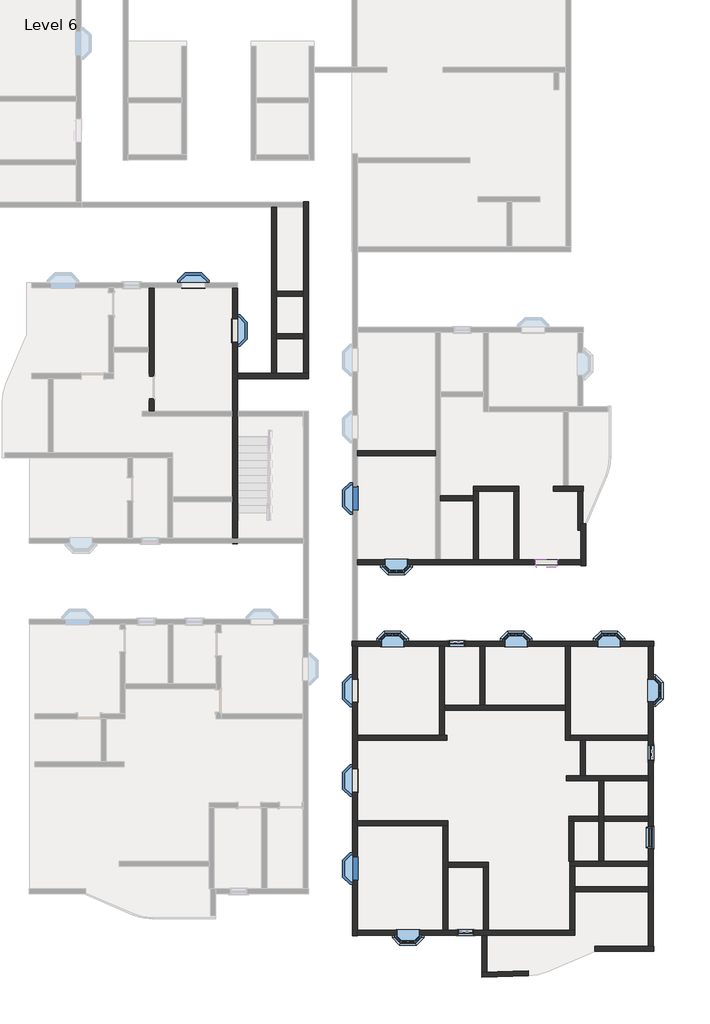
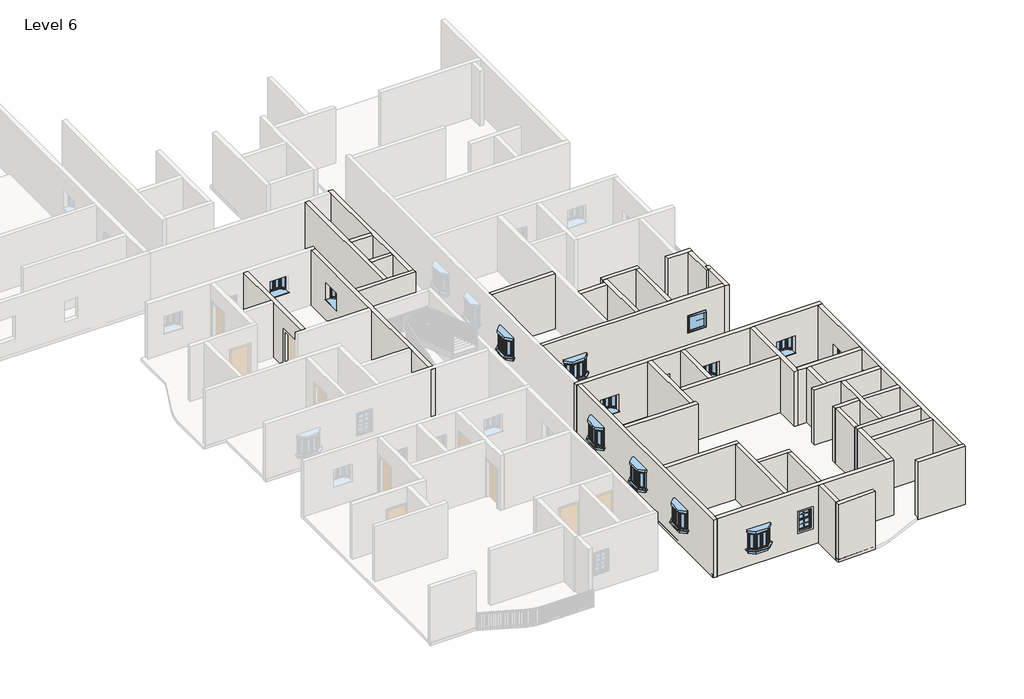
# One storey, part 2 of 14: 41 walls, 17 windows.
"""IFC4 building model written with IfcOpenShell, lengths in millimetres."""

from ifc_helpers import new_model, si_unit, frame, origin, place, context, project, spatial, polyline, outline, extrude, faceted_brep, transform, mapped, element, save
from components import window_910x910mm_67ef725a, window_8debb0fa, windows_sgl_w_glazing_bars_910x910mm_256712d0

model = new_model("IFC4")

# Units and contexts
model_context = context("Model", 3, world=origin())
ifc_project = project(units=[si_unit("LENGTHUNIT", "METRE", prefix="MILLI")], contexts=[model_context])

# Site, building, storey
site = spatial("IfcSite", under=ifc_project)
building = spatial("IfcBuilding", under=site)
storey = spatial("IfcBuildingStorey", under=building, Name="Level 6", Elevation=15240.0)

# Walls
placement = place(None, origin())
element("IfcWall", 1, ObjectType="4.5\" p", at=placement, inside=storey, context=model_context, shape_type="SweptSolid", body=[
    extrude(outline(polyline([(6070.4380523, -28284.6234353), (6070.4380523, -26796.6042694), (6273.6380523, -26796.6042694), (6273.6380523, -28277.5275349), (6070.4380523, -28284.6234353)])), frame((0.0, 0.0, 15240.0), z_axis=(0.0, 0.0, 1.0), x_axis=(1.0, 0.0, 0.0)), (0.0, 0.0, 1.0), 3048.0),
])
element("IfcWall", 2, ObjectType="4.5\" p", at=placement, inside=storey, context=model_context, shape_type="Brep", body=[
    faceted_brep([(6070.4380523, -28487.9472947, 15240.0), (7954.8443294, -28422.1423774, 15240.0), (7954.8443294, -28422.1423774, 18288.0), (6070.4380523, -28487.9472947, 18288.0), (6070.4380523, -28284.6234353, 15240.0), (6070.4380523, -28284.6234353, 18288.0), (6273.6380523, -28277.5275349, 18288.0), (7947.7527517, -28219.0661614, 18288.0), (7947.7527517, -28219.0661614, 15240.0), (6273.6380523, -28277.5275349, 15240.0)], [[[0, 1, 2, 3]], [[4, 5, 6, 7, 8, 9]], [[1, 0, 4, 9, 8]], [[2, 1, 8, 7]], [[3, 2, 7, 6, 5]], [[0, 3, 5, 4]]]),
])
element("IfcWall", 3, ObjectType="4.5\" p", at=placement, inside=storey, context=model_context, shape_type="Brep", body=[
    faceted_brep([(10639.6896214, -27431.6042694, 15240.0), (13030.0380523, -27431.6042694, 15240.0), (13030.0380523, -27431.6042694, 18288.0), (10639.6896214, -27431.6042694, 18288.0), (10639.6896214, -27228.4042694, 15240.0), (10639.6896214, -27228.4042694, 18288.0), (12814.1380523, -27228.4042694, 18288.0), (13017.3380523, -27228.4042694, 18288.0), (13030.0380523, -27228.4042694, 18288.0), (13030.0380523, -27228.4042694, 15240.0), (13017.3380523, -27228.4042694, 15240.0), (12814.1380523, -27228.4042694, 15240.0)], [[[0, 1, 2, 3]], [[4, 5, 6, 7, 8, 9, 10, 11]], [[1, 0, 4, 11, 10, 9]], [[2, 1, 9, 8]], [[3, 2, 8, 7, 6, 5]], [[0, 3, 5, 4]]]),
])
element("IfcWall", 4, ObjectType="4.5\" p", at=placement, inside=storey, context=model_context, shape_type="Brep", body=[
    faceted_brep([(1015.8380523, -18878.1542694, 15240.0), (4648.0380523, -18878.1542694, 15240.0), (4648.0380523, -18878.1542694, 18288.0), (1015.8380523, -18878.1542694, 18288.0), (1015.8380523, -18674.9542694, 15240.0), (1015.8380523, -18674.9542694, 18288.0), (4336.8880523, -18674.9542694, 18288.0), (4540.0880523, -18674.9542694, 18288.0), (4648.0380523, -18674.9542694, 18288.0), (4648.0380523, -18674.9542694, 15240.0), (4540.0880523, -18674.9542694, 15240.0), (4336.8880523, -18674.9542694, 15240.0)], [[[0, 1, 2, 3]], [[4, 5, 6, 7, 8, 9, 10, 11]], [[1, 0, 4, 11, 10, 9]], [[2, 1, 9, 8]], [[3, 2, 8, 7, 6, 5]], [[0, 3, 5, 4]]]),
])
element("IfcWall", 5, ObjectType="4.5\" p", at=placement, inside=storey, context=model_context, shape_type="Brep", body=[
    faceted_brep([(4336.8880523, -15049.1042694, 15240.0), (4336.8880523, -18674.9542694, 15240.0), (4336.8880523, -18674.9542694, 18288.0), (4336.8880523, -15049.1042694, 18288.0), (4540.0880523, -15049.1042694, 15240.0), (4540.0880523, -15049.1042694, 18288.0), (4540.0880523, -17455.7542694, 18288.0), (4540.0880523, -17658.9542694, 18288.0), (4540.0880523, -18674.9542694, 18288.0), (4540.0880523, -18674.9542694, 15240.0), (4540.0880523, -17658.9542694, 15240.0), (4540.0880523, -17455.7542694, 15240.0)], [[[0, 1, 2, 3]], [[4, 5, 6, 7, 8, 9, 10, 11]], [[1, 0, 4, 11, 10, 9]], [[3, 2, 8, 7, 6, 5]], [[0, 3, 5, 4]], [[2, 1, 9, 8]]]),
])
element("IfcWall", 6, ObjectType="4.5\" p", at=placement, inside=storey, context=model_context, shape_type="Brep", body=[
    faceted_brep([(4540.0880523, -17658.9542694, 15240.0), (9442.2880523, -17658.9542694, 15240.0), (9442.2880523, -17658.9542694, 18288.0), (4540.0880523, -17658.9542694, 18288.0), (4540.0880523, -17455.7542694, 15240.0), (4540.0880523, -17455.7542694, 18288.0), (5975.1880523, -17455.7542694, 18288.0), (6178.3880523, -17455.7542694, 18288.0), (9442.2880523, -17455.7542694, 18288.0), (9442.2880523, -17455.7542694, 15240.0), (6178.3880523, -17455.7542694, 15240.0), (5975.1880523, -17455.7542694, 15240.0)], [[[0, 1, 2, 3]], [[4, 5, 6, 7, 8, 9, 10, 11]], [[1, 0, 4, 11, 10, 9]], [[3, 2, 8, 7, 6, 5]], [[0, 3, 5, 4]], [[2, 1, 9, 8]]]),
])
element("IfcWall", 7, ObjectType="4.5\" p", at=placement, inside=storey, context=model_context, shape_type="SweptSolid", body=[
    extrude(outline(polyline([(5975.1880523, -17455.7542694), (5975.1880523, -15049.1042694), (6178.3880523, -15049.1042694), (6178.3880523, -17455.7542694), (5975.1880523, -17455.7542694)])), frame((0.0, 0.0, 15240.0), z_axis=(0.0, 0.0, 1.0), x_axis=(1.0, 0.0, 0.0)), (0.0, 0.0, 1.0), 3048.0),
])
element("IfcWall", 8, ObjectType="4.5\" p", at=placement, inside=storey, context=model_context, shape_type="Brep", body=[
    faceted_brep([(9442.2880523, -15049.1042694, 15240.0), (9442.2880523, -17455.7542694, 15240.0), (9442.2880523, -17658.9542694, 15240.0), (9442.2880523, -18871.8042694, 15240.0), (9442.2880523, -18871.8042694, 18288.0), (9442.2880523, -17658.9542694, 18288.0), (9442.2880523, -17455.7542694, 18288.0), (9442.2880523, -15049.1042694, 18288.0), (9645.4880523, -15049.1042694, 15240.0), (9645.4880523, -15049.1042694, 18288.0), (9645.4880523, -18668.6042694, 18288.0), (9645.4880523, -18871.8042694, 18288.0), (9645.4880523, -18871.8042694, 15240.0), (9645.4880523, -18668.6042694, 15240.0)], [[[0, 1, 2, 3, 4, 5, 6, 7]], [[8, 9, 10, 11, 12, 13]], [[3, 2, 1, 0, 8, 13, 12]], [[7, 6, 5, 4, 11, 10, 9]], [[0, 7, 9, 8]], [[4, 3, 12, 11]]]),
])
element("IfcWall", 9, ObjectType="4.5\" p", at=placement, inside=storey, context=model_context, shape_type="Brep", body=[
    faceted_brep([(1015.8380523, -22345.2542694, 15240.0), (4489.2880523, -22345.2542694, 15240.0), (4692.4880523, -22345.2542694, 15240.0), (4692.4880523, -22345.2542694, 18288.0), (4489.2880523, -22345.2542694, 18288.0), (1015.8380523, -22345.2542694, 18288.0), (1015.8380523, -22142.0542694, 15240.0), (1015.8380523, -22142.0542694, 18288.0), (4692.4880523, -22142.0542694, 18288.0), (4692.4880523, -22142.0542694, 15240.0)], [[[0, 1, 2, 3, 4, 5]], [[6, 7, 8, 9]], [[2, 1, 0, 6, 9]], [[5, 4, 3, 8, 7]], [[0, 5, 7, 6]], [[3, 2, 9, 8]]]),
])
element("IfcWall", 10, ObjectType="4.5\" p", at=placement, inside=storey, context=model_context, shape_type="Brep", body=[
    faceted_brep([(4489.2880523, -22345.2542694, 15240.0), (4489.2880523, -26580.7042694, 15240.0), (4489.2880523, -26580.7042694, 18288.0), (4489.2880523, -22345.2542694, 18288.0), (4692.4880523, -22345.2542694, 15240.0), (4692.4880523, -22345.2542694, 18288.0), (4692.4880523, -23818.4542694, 18288.0), (4692.4880523, -24021.6542694, 18288.0), (4692.4880523, -26580.7042694, 18288.0), (4692.4880523, -26580.7042694, 15240.0), (4692.4880523, -24021.6542694, 15240.0), (4692.4880523, -23818.4542694, 15240.0)], [[[0, 1, 2, 3]], [[4, 5, 6, 7, 8, 9, 10, 11]], [[1, 0, 4, 11, 10, 9]], [[3, 2, 8, 7, 6, 5]], [[0, 3, 5, 4]], [[2, 1, 9, 8]]]),
])
element("IfcWall", 11, ObjectType="4.5\" p", at=placement, inside=storey, context=model_context, shape_type="Brep", body=[
    faceted_brep([(4692.4880523, -24021.6542694, 15240.0), (6127.5880523, -24021.6542694, 15240.0), (6330.7880523, -24021.6542694, 15240.0), (6330.7880523, -24021.6542694, 18288.0), (6127.5880523, -24021.6542694, 18288.0), (4692.4880523, -24021.6542694, 18288.0), (4692.4880523, -23818.4542694, 15240.0), (4692.4880523, -23818.4542694, 18288.0), (6330.7880523, -23818.4542694, 18288.0), (6330.7880523, -23818.4542694, 15240.0)], [[[0, 1, 2, 3, 4, 5]], [[6, 7, 8, 9]], [[2, 1, 0, 6, 9]], [[5, 4, 3, 8, 7]], [[0, 5, 7, 6]], [[3, 2, 9, 8]]]),
])
element("IfcWall", 12, ObjectType="4.5\" p", at=placement, inside=storey, context=model_context, shape_type="SweptSolid", body=[
    extrude(outline(polyline([(6127.5880523, -26580.7042694), (6127.5880523, -24021.6542694), (6330.7880523, -24021.6542694), (6330.7880523, -26580.7042694), (6127.5880523, -26580.7042694)])), frame((0.0, 0.0, 15240.0), z_axis=(0.0, 0.0, 1.0), x_axis=(1.0, 0.0, 0.0)), (0.0, 0.0, 1.0), 3048.0),
])
element("IfcWall", 13, ObjectType="4.5\" p", at=placement, inside=storey, context=model_context, shape_type="Brep", body=[
    faceted_brep([(9645.4880523, -18871.8042694, 15240.0), (10051.8880523, -18871.8042694, 15240.0), (10255.0880523, -18871.8042694, 15240.0), (12814.1380523, -18871.8042694, 15240.0), (12814.1380523, -18871.8042694, 18288.0), (10255.0880523, -18871.8042694, 18288.0), (10051.8880523, -18871.8042694, 18288.0), (9645.4880523, -18871.8042694, 18288.0), (9645.4880523, -18668.6042694, 15240.0), (9645.4880523, -18668.6042694, 18288.0), (12814.1380523, -18668.6042694, 18288.0), (12814.1380523, -18668.6042694, 15240.0)], [[[0, 1, 2, 3, 4, 5, 6, 7]], [[8, 9, 10, 11]], [[3, 2, 1, 0, 8, 11]], [[7, 6, 5, 4, 10, 9]], [[0, 7, 9, 8]], [[4, 3, 11, 10]]]),
])
element("IfcWall", 14, ObjectType="4.5\" p", at=placement, inside=storey, context=model_context, shape_type="SweptSolid", body=[
    extrude(outline(polyline([(10051.8880523, -20313.2542694), (10051.8880523, -18871.8042694), (10255.0880523, -18871.8042694), (10255.0880523, -20313.2542694), (10051.8880523, -20313.2542694)])), frame((0.0, 0.0, 15240.0), z_axis=(0.0, 0.0, 1.0), x_axis=(1.0, 0.0, 0.0)), (0.0, 0.0, 1.0), 3048.0),
])
element("IfcWall", 15, ObjectType="4.5\" p", at=placement, inside=storey, context=model_context, shape_type="Brep", body=[
    faceted_brep([(12814.1380523, -20313.2542694, 15240.0), (10255.0880523, -20313.2542694, 15240.0), (10051.8880523, -20313.2542694, 15240.0), (9486.7380523, -20313.2542694, 15240.0), (9486.7380523, -20313.2542694, 18288.0), (10051.8880523, -20313.2542694, 18288.0), (10255.0880523, -20313.2542694, 18288.0), (12814.1380523, -20313.2542694, 18288.0), (12814.1380523, -20516.4542694, 15240.0), (12814.1380523, -20516.4542694, 18288.0), (11017.0880523, -20516.4542694, 18288.0), (10813.8880523, -20516.4542694, 18288.0), (9486.7380523, -20516.4542694, 18288.0), (9486.7380523, -20516.4542694, 15240.0), (10813.8880523, -20516.4542694, 15240.0), (11017.0880523, -20516.4542694, 15240.0)], [[[0, 1, 2, 3, 4, 5, 6, 7]], [[8, 9, 10, 11, 12, 13, 14, 15]], [[3, 2, 1, 0, 8, 15, 14, 13]], [[4, 3, 13, 12]], [[7, 6, 5, 4, 12, 11, 10, 9]], [[0, 7, 9, 8]]]),
])
element("IfcWall", 16, ObjectType="4.5\" p", at=placement, inside=storey, context=model_context, shape_type="Brep", body=[
    faceted_brep([(10813.8880523, -20516.4542694, 15240.0), (10813.8880523, -21951.5542694, 15240.0), (10813.8880523, -22154.7542694, 15240.0), (10813.8880523, -23779.5416506, 15240.0), (10813.8880523, -23779.5416506, 18288.0), (10813.8880523, -22154.7542694, 18288.0), (10813.8880523, -21951.5542694, 18288.0), (10813.8880523, -20516.4542694, 18288.0), (11017.0880523, -20516.4542694, 15240.0), (11017.0880523, -20516.4542694, 18288.0), (11017.0880523, -21951.5542694, 18288.0), (11017.0880523, -22154.7542694, 18288.0), (11017.0880523, -23779.5416506, 18288.0), (11017.0880523, -23779.5416506, 15240.0), (11017.0880523, -22154.7542694, 15240.0), (11017.0880523, -21951.5542694, 15240.0)], [[[0, 1, 2, 3, 4, 5, 6, 7]], [[8, 9, 10, 11, 12, 13, 14, 15]], [[3, 2, 1, 0, 8, 15, 14, 13]], [[7, 6, 5, 4, 12, 11, 10, 9]], [[0, 7, 9, 8]], [[4, 3, 13, 12]]]),
])
element("IfcWall", 17, ObjectType="4.5\" p", at=placement, inside=storey, context=model_context, shape_type="Brep", body=[
    faceted_brep([(12814.1380523, -23779.5416506, 15240.0), (11017.0880523, -23779.5416506, 15240.0), (10813.8880523, -23779.5416506, 15240.0), (9791.5380523, -23779.5416506, 15240.0), (9632.7880523, -23779.5416506, 15240.0), (9632.7880523, -23779.5416506, 18288.0), (9791.5380523, -23779.5416506, 18288.0), (10813.8880523, -23779.5416506, 18288.0), (11017.0880523, -23779.5416506, 18288.0), (12814.1380523, -23779.5416506, 18288.0), (12814.1380523, -23982.7416506, 15240.0), (12814.1380523, -23982.7416506, 18288.0), (9835.9880523, -23982.7416506, 18288.0), (9632.7880523, -23982.7416506, 18288.0), (9632.7880523, -23982.7416506, 15240.0), (9835.9880523, -23982.7416506, 15240.0)], [[[0, 1, 2, 3, 4, 5, 6, 7, 8, 9]], [[10, 11, 12, 13, 14, 15]], [[4, 3, 2, 1, 0, 10, 15, 14]], [[9, 8, 7, 6, 5, 13, 12, 11]], [[0, 9, 11, 10]], [[5, 4, 14, 13]]]),
])
element("IfcWall", 18, ObjectType="4.5\" p", at=placement, inside=storey, context=model_context, shape_type="Brep", body=[
    faceted_brep([(9632.7880523, -23982.7416506, 15240.0), (9632.7880523, -26580.7042694, 15240.0), (9632.7880523, -26580.7042694, 18288.0), (9632.7880523, -23982.7416506, 18288.0), (9835.9880523, -23982.7416506, 15240.0), (9835.9880523, -23982.7416506, 18288.0), (9835.9880523, -24805.3496998, 18288.0), (9835.9880523, -25008.5496998, 18288.0), (9835.9880523, -26580.7042694, 18288.0), (9835.9880523, -26580.7042694, 15240.0), (9835.9880523, -25008.5496998, 15240.0), (9835.9880523, -24805.3496998, 15240.0)], [[[0, 1, 2, 3]], [[4, 5, 6, 7, 8, 9, 10, 11]], [[1, 0, 4, 11, 10, 9]], [[3, 2, 8, 7, 6, 5]], [[2, 1, 9, 8]], [[0, 3, 5, 4]]]),
])
element("IfcWall", 19, ObjectType="4.5\" p", at=placement, inside=storey, context=model_context, shape_type="SweptSolid", body=[
    extrude(outline(polyline([(12814.1380523, -25008.5496998), (9835.9880523, -25008.5496998), (9835.9880523, -24805.3496998), (12814.1380523, -24805.3496998), (12814.1380523, -25008.5496998)])), frame((0.0, 0.0, 15240.0), z_axis=(0.0, 0.0, 1.0), x_axis=(1.0, 0.0, 0.0)), (0.0, 0.0, 1.0), 3048.0),
])
element("IfcWall", 20, ObjectType="4.5\" p", at=placement, inside=storey, context=model_context, shape_type="Brep", body=[
    faceted_brep([(-7432.737215, -5015.2916506, 17373.6), (-7432.737215, -5015.2916506, 15240.0), (-7432.737215, -5523.2916506, 15240.0), (-7432.737215, -5523.2916506, 18288.0), (-7432.737215, -3135.6916506, 18288.0), (-7432.737215, -2932.4916506, 18288.0), (-7432.737215, -525.8416506, 18288.0), (-7432.737215, -525.8416506, 15240.0), (-7432.737215, -2932.4916506, 15240.0), (-7432.737215, -3135.6916506, 15240.0), (-7432.737215, -4100.8916506, 15240.0), (-7432.737215, -4100.8916506, 17373.6), (-7229.537215, -5523.2916506, 15240.0), (-7229.537215, -5015.2916506, 15240.0), (-7229.537215, -5015.2916506, 17373.6), (-7229.537215, -4100.8916506, 17373.6), (-7229.537215, -4100.8916506, 15240.0), (-7229.537215, -525.8416506, 15240.0), (-7229.537215, -525.8416506, 18288.0), (-7229.537215, -5523.2916506, 18288.0)], [[[0, 1, 2, 3, 4, 5, 6, 7, 8, 9, 10, 11]], [[12, 13, 14, 15, 16, 17, 18, 19]], [[2, 1, 13, 12]], [[10, 9, 8, 7, 17, 16]], [[6, 5, 4, 3, 19, 18]], [[7, 6, 18, 17]], [[3, 2, 12, 19]], [[14, 13, 1, 0]], [[15, 14, 0, 11]], [[16, 15, 11, 10]]]),
])
element("IfcWall", 21, ObjectType="4.5\" p", at=placement, inside=storey, context=model_context, shape_type="Brep", body=[
    faceted_brep([(-3857.687215, -4202.4916506, 15240.0), (-961.4891351, -4202.4916506, 15240.0), (-961.4891351, -4202.4916506, 18288.0), (-3857.687215, -4202.4916506, 18288.0), (-3857.687215, -3999.2916506, 15240.0), (-3857.687215, -3999.2916506, 18288.0), (-2472.7891351, -3999.2916506, 18288.0), (-2269.5891351, -3999.2916506, 18288.0), (-1177.3891351, -3999.2916506, 18288.0), (-974.1891351, -3999.2916506, 18288.0), (-961.4891351, -3999.2916506, 18288.0), (-961.4891351, -3999.2916506, 15240.0), (-974.1891351, -3999.2916506, 15240.0), (-1177.3891351, -3999.2916506, 15240.0), (-2269.5891351, -3999.2916506, 15240.0), (-2472.7891351, -3999.2916506, 15240.0)], [[[0, 1, 2, 3]], [[4, 5, 6, 7, 8, 9, 10, 11, 12, 13, 14, 15]], [[1, 0, 4, 15, 14, 13, 12, 11]], [[2, 1, 11, 10]], [[3, 2, 10, 9, 8, 7, 6, 5]], [[0, 3, 5, 4]]]),
])
element("IfcWall", 22, ObjectType="4.5\" p", at=placement, inside=storey, context=model_context, shape_type="SweptSolid", body=[
    extrude(outline(polyline([(-1177.3891351, -868.7416506), (-2269.5891351, -868.7416506), (-2269.5891351, -665.5416506), (-1177.3891351, -665.5416506), (-1177.3891351, -868.7416506)])), frame((0.0, 0.0, 15240.0), z_axis=(0.0, 0.0, 1.0), x_axis=(1.0, 0.0, 0.0)), (0.0, 0.0, 1.0), 3048.0),
])
element("IfcWall", 23, ObjectType="4.5\" p", at=placement, inside=storey, context=model_context, shape_type="SweptSolid", body=[
    extrude(outline(polyline([(-1177.3891351, -2597.8466506), (-2269.5891351, -2597.8466506), (-2269.5891351, -2394.6466506), (-1177.3891351, -2394.6466506), (-1177.3891351, -2597.8466506)])), frame((0.0, 0.0, 15240.0), z_axis=(0.0, 0.0, 1.0), x_axis=(1.0, 0.0, 0.0)), (0.0, 0.0, 1.0), 3048.0),
])
element("IfcWall", 24, ObjectType="4.5\" p", at=placement, inside=storey, context=model_context, shape_type="SweptSolid", body=[
    extrude(outline(polyline([(5721.1880523, -9162.6542694), (4387.6880523, -9162.6542694), (4387.6880523, -8959.4542694), (5721.1880523, -8959.4542694), (5721.1880523, -9162.6542694)])), frame((0.0, 0.0, 15240.0), z_axis=(0.0, 0.0, 1.0), x_axis=(1.0, 0.0, 0.0)), (0.0, 0.0, 1.0), 3048.0),
])
element("IfcWall", 25, ObjectType="4.5\" p", at=placement, inside=storey, context=model_context, shape_type="Brep", body=[
    faceted_brep([(5721.1880523, -8781.6542694, 15240.0), (5924.3880523, -8781.6542694, 15240.0), (7359.4880523, -8781.6542694, 15240.0), (7562.6880523, -8781.6542694, 15240.0), (7562.6880523, -8781.6542694, 18288.0), (7359.4880523, -8781.6542694, 18288.0), (5924.3880523, -8781.6542694, 18288.0), (5721.1880523, -8781.6542694, 18288.0), (5721.1880523, -8578.4542694, 15240.0), (5721.1880523, -8578.4542694, 18288.0), (7562.6880523, -8578.4542694, 18288.0), (7562.6880523, -8578.4542694, 15240.0)], [[[0, 1, 2, 3, 4, 5, 6, 7]], [[8, 9, 10, 11]], [[3, 2, 1, 0, 8, 11]], [[7, 6, 5, 4, 10, 9]], [[0, 7, 9, 8]], [[4, 3, 11, 10]]]),
])
element("IfcWall", 26, ObjectType="4.5\" p", at=placement, inside=storey, context=model_context, shape_type="Brep", body=[
    faceted_brep([(5721.1880523, -8781.6542694, 15240.0), (5721.1880523, -8959.4542694, 15240.0), (5721.1880523, -9162.6542694, 15240.0), (5721.1880523, -11556.6042694, 15240.0), (5721.1880523, -11556.6042694, 18288.0), (5721.1880523, -9162.6542694, 18288.0), (5721.1880523, -8959.4542694, 18288.0), (5721.1880523, -8781.6542694, 18288.0), (5924.3880523, -8781.6542694, 15240.0), (5924.3880523, -8781.6542694, 18288.0), (5924.3880523, -11556.6042694, 18288.0), (5924.3880523, -11556.6042694, 15240.0)], [[[0, 1, 2, 3, 4, 5, 6, 7]], [[8, 9, 10, 11]], [[3, 2, 1, 0, 8, 11]], [[7, 6, 5, 4, 10, 9]], [[0, 7, 9, 8]], [[4, 3, 11, 10]]]),
])
element("IfcWall", 27, ObjectType="4.5\" p", at=placement, inside=storey, context=model_context, shape_type="SweptSolid", body=[
    extrude(outline(polyline([(7359.4880523, -11556.6042694), (7359.4880523, -8781.6542694), (7562.6880523, -8781.6542694), (7562.6880523, -11556.6042694), (7359.4880523, -11556.6042694)])), frame((0.0, 0.0, 15240.0), z_axis=(0.0, 0.0, 1.0), x_axis=(1.0, 0.0, 0.0)), (0.0, 0.0, 1.0), 3048.0),
])
element("IfcWall", 28, ObjectType="4.5\" p", at=placement, inside=storey, context=model_context, shape_type="SweptSolid", body=[
    extrude(outline(polyline([(4184.4880523, -7333.8542694), (1007.0108649, -7333.8542694), (1007.0108649, -7130.6542694), (4184.4880523, -7130.6542694), (4184.4880523, -7333.8542694)])), frame((0.0, 0.0, 15240.0), z_axis=(0.0, 0.0, 1.0), x_axis=(1.0, 0.0, 0.0)), (0.0, 0.0, 1.0), 3048.0),
])
element("IfcWall", 29, ObjectType="4.5\" p", at=placement, inside=storey, context=model_context, shape_type="Brep", body=[
    faceted_brep([(8953.3380523, -8781.6542694, 15240.0), (9956.6380523, -8781.6542694, 15240.0), (10159.8380523, -8781.6542694, 15240.0), (10172.5380523, -8781.6542694, 15240.0), (10172.5380523, -8781.6542694, 18288.0), (10159.8380523, -8781.6542694, 18288.0), (9956.6380523, -8781.6542694, 18288.0), (8953.3380523, -8781.6542694, 18288.0), (8953.3380523, -8578.4542694, 15240.0), (8953.3380523, -8578.4542694, 18288.0), (9371.2322031, -8578.4542694, 18288.0), (9574.4322031, -8578.4542694, 18288.0), (10172.5380523, -8578.4542694, 18288.0), (10172.5380523, -8578.4542694, 15240.0), (9574.4322031, -8578.4542694, 15240.0), (9371.2322031, -8578.4542694, 15240.0)], [[[0, 1, 2, 3, 4, 5, 6, 7]], [[8, 9, 10, 11, 12, 13, 14, 15]], [[3, 2, 1, 0, 8, 15, 14, 13]], [[4, 3, 13, 12]], [[7, 6, 5, 4, 12, 11, 10, 9]], [[0, 7, 9, 8]]]),
])
element("IfcWall", 30, ObjectType="4.5\" p", at=placement, inside=storey, context=model_context, shape_type="SweptSolid", body=[
    extrude(outline(polyline([(9956.6380523, -10352.8912671), (9956.6380523, -8781.6542694), (10159.8380523, -8781.6542694), (10159.8380523, -10352.8912671), (9956.6380523, -10352.8912671)])), frame((0.0, 0.0, 15240.0), z_axis=(0.0, 0.0, 1.0), x_axis=(1.0, 0.0, 0.0)), (0.0, 0.0, 1.0), 3048.0),
])
element("IfcWall", 31, ObjectType="4.5\" p", at=placement, inside=storey, context=model_context, shape_type="Brep", body=[
    faceted_brep([(12814.1380523, -21951.5542694, 18288.0), (12814.1380523, -21951.5542694, 15240.0), (11017.0880523, -21951.5542694, 15240.0), (11017.0880523, -21951.5542694, 18288.0), (12814.1380523, -22154.7542694, 15240.0), (12814.1380523, -22154.7542694, 18288.0), (11017.0880523, -22154.7542694, 18288.0), (11017.0880523, -22154.7542694, 15240.0)], [[[0, 1, 2, 3]], [[4, 5, 6, 7]], [[1, 4, 7, 2]], [[5, 0, 3, 6]], [[1, 0, 5, 4]], [[3, 2, 7, 6]]]),
    faceted_brep([(9588.3380523, -21951.5542694, 15240.0), (9588.3380523, -21951.5542694, 18288.0), (10813.8880523, -21951.5542694, 18288.0), (10813.8880523, -21951.5542694, 15240.0), (9588.3380523, -22154.7542694, 18288.0), (9588.3380523, -22154.7542694, 15240.0), (9791.5380523, -22154.7542694, 15240.0), (10813.8880523, -22154.7542694, 15240.0), (10813.8880523, -22154.7542694, 18288.0), (9791.5380523, -22154.7542694, 18288.0)], [[[0, 1, 2, 3]], [[4, 5, 6, 7, 8, 9]], [[5, 0, 3, 7, 6]], [[1, 4, 9, 8, 2]], [[3, 2, 8, 7]], [[1, 0, 5, 4]]]),
])
element("IfcWall", 32, ObjectType="4.5\" p", at=placement, inside=storey, context=model_context, shape_type="Brep", body=[
    faceted_brep([(9588.3380523, -22154.7542694, 15240.0), (9588.3380523, -23779.5416506, 15240.0), (9588.3380523, -23779.5416506, 18288.0), (9588.3380523, -22154.7542694, 18288.0), (9791.5380523, -22154.7542694, 15240.0), (9791.5380523, -22154.7542694, 18288.0), (9791.5380523, -23779.5416506, 18288.0), (9791.5380523, -23779.5416506, 15240.0), (9632.7880523, -23779.5416506, 15240.0), (9632.7880523, -23779.5416506, 18288.0)], [[[0, 1, 2, 3]], [[4, 5, 6, 7]], [[1, 0, 4, 7, 8]], [[3, 2, 9, 6, 5]], [[2, 1, 8, 7, 6, 9]], [[0, 3, 5, 4]]]),
])
element("IfcWall", 33, ObjectType="9\"", at=placement, inside=storey, context=model_context, shape_type="Brep", body=[
    faceted_brep([(799.9380523, -15049.1042694, 15240.0), (812.6380523, -15049.1042694, 15240.0), (1015.8380523, -15049.1042694, 15240.0), (4336.8880523, -15049.1042694, 15240.0), (4540.0880523, -15049.1042694, 15240.0), (5975.1880523, -15049.1042694, 15240.0), (6178.3880523, -15049.1042694, 15240.0), (9442.2880523, -15049.1042694, 15240.0), (9645.4880523, -15049.1042694, 15240.0), (12814.1380523, -15049.1042694, 15240.0), (13017.3380523, -15049.1042694, 15240.0), (13030.0380523, -15049.1042694, 15240.0), (13030.0380523, -15049.1042694, 18288.0), (13017.3380523, -15049.1042694, 18288.0), (12814.1380523, -15049.1042694, 18288.0), (9645.4880523, -15049.1042694, 18288.0), (9442.2880523, -15049.1042694, 18288.0), (6178.3880523, -15049.1042694, 18288.0), (5975.1880523, -15049.1042694, 18288.0), (4540.0880523, -15049.1042694, 18288.0), (4336.8880523, -15049.1042694, 18288.0), (1015.8380523, -15049.1042694, 18288.0), (812.6380523, -15049.1042694, 18288.0), (799.9380523, -15049.1042694, 18288.0), (1983.2380523, -15049.1042694, 17064.4), (2893.2380523, -15049.1042694, 17064.4), (2893.2380523, -15049.1042694, 16154.4), (1983.2380523, -15049.1042694, 16154.4), (10774.8130523, -15049.1042694, 17064.4), (11684.8130523, -15049.1042694, 17064.4), (11684.8130523, -15049.1042694, 16154.4), (10774.8130523, -15049.1042694, 16154.4), (6993.3880523, -15049.1042694, 17064.4), (7903.3880523, -15049.1042694, 17064.4), (7903.3880523, -15049.1042694, 16154.4), (6993.3880523, -15049.1042694, 16154.4), (4717.8880523, -15049.1042694, 17221.2), (5378.2880523, -15049.1042694, 17221.2), (5378.2880523, -15049.1042694, 16154.4), (4717.8880523, -15049.1042694, 16154.4), (799.9380523, -14845.9042694, 15240.0), (799.9380523, -14845.9042694, 18288.0), (803.8108649, -14845.9042694, 18288.0), (1007.0108649, -14845.9042694, 18288.0), (13030.0380523, -14845.9042694, 18288.0), (13030.0380523, -14845.9042694, 15240.0), (1007.0108649, -14845.9042694, 15240.0), (803.8108649, -14845.9042694, 15240.0), (1983.2380523, -14845.9042694, 17064.4), (1983.2380523, -14845.9042694, 16154.4), (2893.2380523, -14845.9042694, 16154.4), (2893.2380523, -14845.9042694, 17064.4), (10774.8130523, -14845.9042694, 17064.4), (10774.8130523, -14845.9042694, 16154.4), (11684.8130523, -14845.9042694, 16154.4), (11684.8130523, -14845.9042694, 17064.4), (6993.3880523, -14845.9042694, 17064.4), (6993.3880523, -14845.9042694, 16154.4), (7903.3880523, -14845.9042694, 16154.4), (7903.3880523, -14845.9042694, 17064.4), (4717.8880523, -14845.9042694, 17221.2), (4717.8880523, -14845.9042694, 16154.4), (5378.2880523, -14845.9042694, 16154.4), (5378.2880523, -14845.9042694, 17221.2)], [[[0, 1, 2, 3, 4, 5, 6, 7, 8, 9, 10, 11, 12, 13, 14, 15, 16, 17, 18, 19, 20, 21, 22, 23], [24, 25, 26, 27], [28, 29, 30, 31], [32, 33, 34, 35], [36, 37, 38, 39]], [[40, 41, 42, 43, 44, 45, 46, 47], [48, 49, 50, 51], [52, 53, 54, 55], [56, 57, 58, 59], [60, 61, 62, 63]], [[11, 10, 9, 8, 7, 6, 5, 4, 3, 2, 1, 0, 40, 47, 46, 45]], [[12, 11, 45, 44]], [[23, 22, 21, 20, 19, 18, 17, 16, 15, 14, 13, 12, 44, 43, 42, 41]], [[0, 23, 41, 40]], [[49, 48, 24, 27]], [[50, 49, 27, 26]], [[51, 50, 26, 25]], [[48, 51, 25, 24]], [[53, 52, 28, 31]], [[54, 53, 31, 30]], [[55, 54, 30, 29]], [[52, 55, 29, 28]], [[57, 56, 32, 35]], [[58, 57, 35, 34]], [[59, 58, 34, 33]], [[56, 59, 33, 32]], [[61, 60, 36, 39]], [[62, 61, 39, 38]], [[63, 62, 38, 37]], [[60, 63, 37, 36]]]),
])
element("IfcWall", 34, ObjectType="9\"", at=placement, inside=storey, context=model_context, shape_type="Brep", body=[
    faceted_brep([(12814.1380523, -15049.1042694, 15240.0), (12814.1380523, -18668.6042694, 15240.0), (12814.1380523, -18871.8042694, 15240.0), (12814.1380523, -20313.2542694, 15240.0), (12814.1380523, -20516.4542694, 15240.0), (12814.1380523, -21951.5542694, 15240.0), (12814.1380523, -22154.7542694, 15240.0), (12814.1380523, -23779.5416506, 15240.0), (12814.1380523, -23982.7416506, 15240.0), (12814.1380523, -24805.3496998, 15240.0), (12814.1380523, -25008.5496998, 15240.0), (12814.1380523, -27228.4042694, 15240.0), (12814.1380523, -27228.4042694, 18288.0), (12814.1380523, -25008.5496998, 18288.0), (12814.1380523, -24805.3496998, 18288.0), (12814.1380523, -23982.7416506, 18288.0), (12814.1380523, -23779.5416506, 18288.0), (12814.1380523, -22154.7542694, 18288.0), (12814.1380523, -21951.5542694, 18288.0), (12814.1380523, -20516.4542694, 18288.0), (12814.1380523, -20313.2542694, 18288.0), (12814.1380523, -18871.8042694, 18288.0), (12814.1380523, -18668.6042694, 18288.0), (12814.1380523, -15049.1042694, 18288.0), (12814.1380523, -16403.8542694, 17064.4), (12814.1380523, -17313.8542694, 17064.4), (12814.1380523, -17313.8542694, 16154.4), (12814.1380523, -16403.8542694, 16154.4), (12814.1380523, -23270.1542694, 17064.4), (12814.1380523, -23270.1542694, 16154.4), (12814.1380523, -22360.1542694, 16154.4), (12814.1380523, -22360.1542694, 17064.4), (12814.1380523, -19049.6042694, 17221.2), (12814.1380523, -19710.0042694, 17221.2), (12814.1380523, -19710.0042694, 16154.4), (12814.1380523, -19049.6042694, 16154.4), (13017.3380523, -15049.1042694, 15240.0), (13017.3380523, -15049.1042694, 18288.0), (13017.3380523, -27228.4042694, 18288.0), (13017.3380523, -27228.4042694, 15240.0), (13017.3380523, -16403.8542694, 17064.4), (13017.3380523, -16403.8542694, 16154.4), (13017.3380523, -17313.8542694, 16154.4), (13017.3380523, -17313.8542694, 17064.4), (13017.3380523, -23270.1542694, 17064.4), (13017.3380523, -22360.1542694, 17064.4), (13017.3380523, -22360.1542694, 16154.4), (13017.3380523, -23270.1542694, 16154.4), (13017.3380523, -19049.6042694, 17221.2), (13017.3380523, -19049.6042694, 16154.4), (13017.3380523, -19710.0042694, 16154.4), (13017.3380523, -19710.0042694, 17221.2)], [[[0, 1, 2, 3, 4, 5, 6, 7, 8, 9, 10, 11, 12, 13, 14, 15, 16, 17, 18, 19, 20, 21, 22, 23], [24, 25, 26, 27], [28, 29, 30, 31], [32, 33, 34, 35]], [[36, 37, 38, 39], [40, 41, 42, 43], [44, 45, 46, 47], [48, 49, 50, 51]], [[11, 10, 9, 8, 7, 6, 5, 4, 3, 2, 1, 0, 36, 39]], [[23, 22, 21, 20, 19, 18, 17, 16, 15, 14, 13, 12, 38, 37]], [[0, 23, 37, 36]], [[12, 11, 39, 38]], [[41, 40, 24, 27]], [[42, 41, 27, 26]], [[43, 42, 26, 25]], [[40, 43, 25, 24]], [[29, 28, 44, 47]], [[30, 29, 47, 46]], [[31, 30, 46, 45]], [[28, 31, 45, 44]], [[49, 48, 32, 35]], [[50, 49, 35, 34]], [[51, 50, 34, 33]], [[48, 51, 33, 32]]]),
])
element("IfcWall", 35, ObjectType="9\"", at=placement, inside=storey, context=model_context, shape_type="Brep", body=[
    faceted_brep([(812.6380523, -15049.1042694, 15240.0), (812.6380523, -26796.6042694, 15240.0), (812.6380523, -26796.6042694, 18288.0), (812.6380523, -15049.1042694, 18288.0), (812.6380523, -24527.4542694, 17350.0), (812.6380523, -24527.4542694, 16440.0), (812.6380523, -23617.4542694, 16440.0), (812.6380523, -23617.4542694, 17350.0), (812.6380523, -20965.1042694, 17350.0), (812.6380523, -20965.1042694, 16440.0), (812.6380523, -20055.1042694, 16440.0), (812.6380523, -20055.1042694, 17350.0), (812.6380523, -17317.0292694, 17350.0), (812.6380523, -17317.0292694, 16440.0), (812.6380523, -16407.0292694, 16440.0), (812.6380523, -16407.0292694, 17350.0), (1015.8380523, -15049.1042694, 15240.0), (1015.8380523, -15049.1042694, 18288.0), (1015.8380523, -18674.9542694, 18288.0), (1015.8380523, -18878.1542694, 18288.0), (1015.8380523, -22142.0542694, 18288.0), (1015.8380523, -22345.2542694, 18288.0), (1015.8380523, -26580.7042694, 18288.0), (1015.8380523, -26783.9042694, 18288.0), (1015.8380523, -26796.6042694, 18288.0), (1015.8380523, -26796.6042694, 15240.0), (1015.8380523, -26783.9042694, 15240.0), (1015.8380523, -26580.7042694, 15240.0), (1015.8380523, -22345.2542694, 15240.0), (1015.8380523, -22142.0542694, 15240.0), (1015.8380523, -18878.1542694, 15240.0), (1015.8380523, -18674.9542694, 15240.0), (1015.8380523, -24527.4542694, 17350.0), (1015.8380523, -23617.4542694, 17350.0), (1015.8380523, -23617.4542694, 16440.0), (1015.8380523, -24527.4542694, 16440.0), (1015.8380523, -20965.1042694, 17350.0), (1015.8380523, -20055.1042694, 17350.0), (1015.8380523, -20055.1042694, 16440.0), (1015.8380523, -20965.1042694, 16440.0), (1015.8380523, -17317.0292694, 17350.0), (1015.8380523, -16407.0292694, 17350.0), (1015.8380523, -16407.0292694, 16440.0), (1015.8380523, -17317.0292694, 16440.0)], [[[0, 1, 2, 3], [4, 5, 6, 7], [8, 9, 10, 11], [12, 13, 14, 15]], [[16, 17, 18, 19, 20, 21, 22, 23, 24, 25, 26, 27, 28, 29, 30, 31], [32, 33, 34, 35], [36, 37, 38, 39], [40, 41, 42, 43]], [[1, 0, 16, 31, 30, 29, 28, 27, 26, 25]], [[2, 1, 25, 24]], [[3, 2, 24, 23, 22, 21, 20, 19, 18, 17]], [[0, 3, 17, 16]], [[5, 4, 32, 35]], [[6, 5, 35, 34]], [[7, 6, 34, 33]], [[4, 7, 33, 32]], [[9, 8, 36, 39]], [[10, 9, 39, 38]], [[11, 10, 38, 37]], [[8, 11, 37, 36]], [[13, 12, 40, 43]], [[14, 13, 43, 42]], [[15, 14, 42, 41]], [[12, 15, 41, 40]]]),
])
element("IfcWall", 36, ObjectType="9\"", at=placement, inside=storey, context=model_context, shape_type="Brep", body=[
    faceted_brep([(1015.8380523, -26783.9042694, 15240.0), (9835.9880523, -26783.9042694, 15240.0), (9835.9880523, -26783.9042694, 18288.0), (1015.8380523, -26783.9042694, 18288.0), (3521.8880523, -26783.9042694, 17064.4), (3521.8880523, -26783.9042694, 16154.4), (2611.8880523, -26783.9042694, 16154.4), (2611.8880523, -26783.9042694, 17064.4), (5079.8380523, -26783.9042694, 17221.2), (5740.2380523, -26783.9042694, 17221.2), (5740.2380523, -26783.9042694, 16154.4), (5079.8380523, -26783.9042694, 16154.4), (1015.8380523, -26580.7042694, 15240.0), (1015.8380523, -26580.7042694, 18288.0), (4489.2880523, -26580.7042694, 18288.0), (4692.4880523, -26580.7042694, 18288.0), (6127.5880523, -26580.7042694, 18288.0), (6330.7880523, -26580.7042694, 18288.0), (9632.7880523, -26580.7042694, 18288.0), (9835.9880523, -26580.7042694, 18288.0), (9835.9880523, -26580.7042694, 15240.0), (9632.7880523, -26580.7042694, 15240.0), (6330.7880523, -26580.7042694, 15240.0), (6127.5880523, -26580.7042694, 15240.0), (4692.4880523, -26580.7042694, 15240.0), (4489.2880523, -26580.7042694, 15240.0), (3521.8880523, -26580.7042694, 17064.4), (2611.8880523, -26580.7042694, 17064.4), (2611.8880523, -26580.7042694, 16154.4), (3521.8880523, -26580.7042694, 16154.4), (5079.8380523, -26580.7042694, 17221.2), (5079.8380523, -26580.7042694, 16154.4), (5740.2380523, -26580.7042694, 16154.4), (5740.2380523, -26580.7042694, 17221.2)], [[[0, 1, 2, 3], [4, 5, 6, 7], [8, 9, 10, 11]], [[12, 13, 14, 15, 16, 17, 18, 19, 20, 21, 22, 23, 24, 25], [26, 27, 28, 29], [30, 31, 32, 33]], [[1, 0, 12, 25, 24, 23, 22, 21, 20]], [[3, 2, 19, 18, 17, 16, 15, 14, 13]], [[0, 3, 13, 12]], [[2, 1, 20, 19]], [[5, 4, 26, 29]], [[6, 5, 29, 28]], [[7, 6, 28, 27]], [[4, 7, 27, 26]], [[31, 30, 8, 11]], [[32, 31, 11, 10]], [[33, 32, 10, 9]], [[30, 33, 9, 8]]]),
])
element("IfcWall", 37, ObjectType="9\" w", at=placement, inside=storey, context=model_context, shape_type="Brep", body=[
    faceted_brep([(-4060.887215, -525.8416506, 15240.0), (-4060.887215, -5523.2916506, 15240.0), (-4060.887215, -5726.4916506, 15240.0), (-4060.887215, -8990.3916506, 15240.0), (-4060.887215, -9193.5916506, 15240.0), (-4060.887215, -10901.7416506, 15240.0), (-4060.887215, -10901.7416506, 18288.0), (-4060.887215, -9193.5916506, 18288.0), (-4060.887215, -8990.3916506, 18288.0), (-4060.887215, -5726.4916506, 18288.0), (-4060.887215, -5523.2916506, 18288.0), (-4060.887215, -525.8416506, 18288.0), (-4060.887215, -1807.5666506, 17350.0), (-4060.887215, -2717.5666506, 17350.0), (-4060.887215, -2717.5666506, 16440.0), (-4060.887215, -1807.5666506, 16440.0), (-3857.687215, -525.8416506, 15240.0), (-3857.687215, -525.8416506, 18288.0), (-3857.687215, -3999.2916506, 18288.0), (-3857.687215, -4202.4916506, 18288.0), (-3857.687215, -5523.2916506, 18288.0), (-3857.687215, -5726.4916506, 18288.0), (-3857.687215, -10901.7416506, 18288.0), (-3857.687215, -10901.7416506, 15240.0), (-3857.687215, -5726.4916506, 15240.0), (-3857.687215, -5523.2916506, 15240.0), (-3857.687215, -4202.4916506, 15240.0), (-3857.687215, -3999.2916506, 15240.0), (-3857.687215, -1807.5666506, 17350.0), (-3857.687215, -1807.5666506, 16440.0), (-3857.687215, -2717.5666506, 16440.0), (-3857.687215, -2717.5666506, 17350.0)], [[[0, 1, 2, 3, 4, 5, 6, 7, 8, 9, 10, 11], [12, 13, 14, 15]], [[16, 17, 18, 19, 20, 21, 22, 23, 24, 25, 26, 27], [28, 29, 30, 31]], [[5, 4, 3, 2, 1, 0, 16, 27, 26, 25, 24, 23]], [[6, 5, 23, 22]], [[11, 10, 9, 8, 7, 6, 22, 21, 20, 19, 18, 17]], [[0, 11, 17, 16]], [[29, 28, 12, 15]], [[30, 29, 15, 14]], [[31, 30, 14, 13]], [[28, 31, 13, 12]]]),
])
element("IfcWall", 38, ObjectType="9\" w", at=placement, inside=storey, context=model_context, shape_type="Brep", body=[
    faceted_brep([(-2269.5891351, -3999.2916506, 15240.0), (-2269.5891351, -2597.8466506, 15240.0), (-2269.5891351, -2394.6466506, 15240.0), (-2269.5891351, -868.7416506, 15240.0), (-2269.5891351, -665.5416506, 15240.0), (-2269.5891351, 2750.7583494, 15240.0), (-2269.5891351, 2750.7583494, 18288.0), (-2269.5891351, -665.5416506, 18288.0), (-2269.5891351, -868.7416506, 18288.0), (-2269.5891351, -2394.6466506, 18288.0), (-2269.5891351, -2597.8466506, 18288.0), (-2269.5891351, -3999.2916506, 18288.0), (-2472.7891351, -3999.2916506, 15240.0), (-2472.7891351, -3999.2916506, 18288.0), (-2472.7891351, 2750.7583494, 18288.0), (-2472.7891351, 2750.7583494, 15240.0)], [[[0, 1, 2, 3, 4, 5, 6, 7, 8, 9, 10, 11]], [[12, 13, 14, 15]], [[5, 4, 3, 2, 1, 0, 12, 15]], [[11, 10, 9, 8, 7, 6, 14, 13]], [[0, 11, 13, 12]], [[6, 5, 15, 14]]]),
])
element("IfcWall", 39, ObjectType="9\" w", at=placement, inside=storey, context=model_context, shape_type="Brep", body=[
    faceted_brep([(-974.1891351, -3999.2916506, 15240.0), (-974.1891351, 2966.6583494, 15240.0), (-974.1891351, 2966.6583494, 18288.0), (-974.1891351, -3999.2916506, 18288.0), (-1177.3891351, -3999.2916506, 15240.0), (-1177.3891351, -3999.2916506, 18288.0), (-1177.3891351, -2597.8466506, 18288.0), (-1177.3891351, -2394.6466506, 18288.0), (-1177.3891351, -868.7416506, 18288.0), (-1177.3891351, -665.5416506, 18288.0), (-1177.3891351, 2750.7583494, 18288.0), (-1177.3891351, 2953.9583494, 18288.0), (-1177.3891351, 2966.6583494, 18288.0), (-1177.3891351, 2966.6583494, 15240.0), (-1177.3891351, 2953.9583494, 15240.0), (-1177.3891351, 2750.7583494, 15240.0), (-1177.3891351, -665.5416506, 15240.0), (-1177.3891351, -868.7416506, 15240.0), (-1177.3891351, -2394.6466506, 15240.0), (-1177.3891351, -2597.8466506, 15240.0)], [[[0, 1, 2, 3]], [[4, 5, 6, 7, 8, 9, 10, 11, 12, 13, 14, 15, 16, 17, 18, 19]], [[1, 0, 4, 19, 18, 17, 16, 15, 14, 13]], [[2, 1, 13, 12]], [[3, 2, 12, 11, 10, 9, 8, 7, 6, 5]], [[0, 3, 5, 4]]]),
])
element("IfcWall", 40, ObjectType="9\" w", at=placement, inside=storey, context=model_context, shape_type="Brep", body=[
    faceted_brep([(1007.0108649, -11759.8042694, 15240.0), (10070.9380523, -11759.8042694, 15240.0), (10070.9380523, -11759.8042694, 18288.0), (1007.0108649, -11759.8042694, 18288.0), (3050.7494586, -11759.8042694, 17064.4), (3050.7494586, -11759.8042694, 16154.4), (2140.7494586, -11759.8042694, 16154.4), (2140.7494586, -11759.8042694, 17064.4), (9135.2880523, -11759.8042694, 17350.0), (9135.2880523, -11759.8042694, 16440.0), (8225.2880523, -11759.8042694, 16440.0), (8225.2880523, -11759.8042694, 17350.0), (1007.0108649, -11556.6042694, 15240.0), (1007.0108649, -11556.6042694, 18288.0), (4184.4880523, -11556.6042694, 18288.0), (4387.6880523, -11556.6042694, 18288.0), (5721.1880523, -11556.6042694, 18288.0), (5924.3880523, -11556.6042694, 18288.0), (7359.4880523, -11556.6042694, 18288.0), (7562.6880523, -11556.6042694, 18288.0), (10070.9380523, -11556.6042694, 18288.0), (10070.9380523, -11556.6042694, 15240.0), (7562.6880523, -11556.6042694, 15240.0), (7359.4880523, -11556.6042694, 15240.0), (5924.3880523, -11556.6042694, 15240.0), (5721.1880523, -11556.6042694, 15240.0), (4387.6880523, -11556.6042694, 15240.0), (4184.4880523, -11556.6042694, 15240.0), (3050.7494586, -11556.6042694, 17064.4), (2140.7494586, -11556.6042694, 17064.4), (2140.7494586, -11556.6042694, 16154.4), (3050.7494586, -11556.6042694, 16154.4), (9135.2880523, -11556.6042694, 17350.0), (8225.2880523, -11556.6042694, 17350.0), (8225.2880523, -11556.6042694, 16440.0), (9135.2880523, -11556.6042694, 16440.0)], [[[0, 1, 2, 3], [4, 5, 6, 7], [8, 9, 10, 11]], [[12, 13, 14, 15, 16, 17, 18, 19, 20, 21, 22, 23, 24, 25, 26, 27], [28, 29, 30, 31], [32, 33, 34, 35]], [[1, 0, 12, 27, 26, 25, 24, 23, 22, 21]], [[3, 2, 20, 19, 18, 17, 16, 15, 14, 13]], [[0, 3, 13, 12]], [[2, 1, 21, 20]], [[5, 4, 28, 31]], [[6, 5, 31, 30]], [[7, 6, 30, 29]], [[4, 7, 29, 28]], [[9, 8, 32, 35]], [[10, 9, 35, 34]], [[11, 10, 34, 33]], [[8, 11, 33, 32]]]),
])
element("IfcWall", 41, ObjectType="9\" w", at=placement, inside=storey, context=model_context, shape_type="Brep", body=[
    faceted_brep([(10070.9380523, -10085.9721442, 15240.0), (10070.9380523, -11556.6042694, 15240.0), (10070.9380523, -11759.8042694, 15240.0), (10070.9380523, -11785.2042694, 15240.0), (10070.9380523, -11785.2042694, 18288.0), (10070.9380523, -11759.8042694, 18288.0), (10070.9380523, -11556.6042694, 18288.0), (10070.9380523, -10085.9721442, 18288.0), (10274.1380523, -10085.9721442, 15240.0), (10274.1380523, -10085.9721442, 18288.0), (10274.1380523, -11785.2042694, 18288.0), (10274.1380523, -11785.2042694, 15240.0)], [[[0, 1, 2, 3, 4, 5, 6, 7]], [[8, 9, 10, 11]], [[3, 2, 1, 0, 8, 11]], [[4, 3, 11, 10]], [[7, 6, 5, 4, 10, 9]], [[0, 7, 9, 8]]]),
])

# Windows
window_910x910mm_shape = window_910x910mm_67ef725a(model_context)
element("IfcWindow", 42, ObjectType="910x910mm", at=placement, inside=storey, context=model_context, shape_type="MappedRepresentation", body=[
    mapped(window_910x910mm_shape, transform((-5075.212215, -432.6982184, 15240.0), x_axis=(1.0, 0.0, 0.0), y_axis=(0.0, 1.0, 0.0), z_axis=(0.0, 0.0, 1.0))),
])
element("IfcWindow", 43, ObjectType="910x910mm", at=placement, inside=storey, context=model_context, shape_type="MappedRepresentation", body=[
    mapped(window_910x910mm_shape, transform((-3967.7437828, -2832.5666506, 15240.0), x_axis=(0.0, -1.0, 0.0), y_axis=(1.0, 0.0, 0.0), z_axis=(0.0, 0.0, 1.0))),
])
element("IfcWindow", 44, ObjectType="910x910mm", at=placement, inside=storey, context=model_context, shape_type="MappedRepresentation", body=[
    mapped(window_910x910mm_shape, transform((2025.7494586, -11649.7477016, 14954.4), x_axis=(-1.0, 0.0, 0.0), y_axis=(0.0, -1.0, 0.0), z_axis=(0.0, 0.0, 1.0))),
])
element("IfcWindow", 45, ObjectType="910x910mm", at=placement, inside=storey, context=model_context, shape_type="MappedRepresentation", body=[
    mapped(window_910x910mm_shape, transform((2496.8880523, -26673.8477016, 14954.4), x_axis=(-1.0, 0.0, 0.0), y_axis=(0.0, -1.0, 0.0), z_axis=(0.0, 0.0, 1.0))),
])
element("IfcWindow", 46, ObjectType="910x910mm", at=placement, inside=storey, context=model_context, shape_type="MappedRepresentation", body=[
    mapped(window_910x910mm_shape, transform((922.6946201, -23502.4542694, 15240.0), x_axis=(0.0, 1.0, 0.0), y_axis=(-1.0, 0.0, 0.0), z_axis=(0.0, 0.0, 1.0))),
])
element("IfcWindow", 47, ObjectType="910x910mm", at=placement, inside=storey, context=model_context, shape_type="MappedRepresentation", body=[
    mapped(window_910x910mm_shape, transform((922.6946201, -19940.1042694, 15240.0), x_axis=(0.0, 1.0, 0.0), y_axis=(-1.0, 0.0, 0.0), z_axis=(0.0, 0.0, 1.0))),
])
element("IfcWindow", 48, ObjectType="910x910mm", at=placement, inside=storey, context=model_context, shape_type="MappedRepresentation", body=[
    mapped(window_910x910mm_shape, transform((922.6946201, -16292.0292694, 15240.0), x_axis=(0.0, 1.0, 0.0), y_axis=(-1.0, 0.0, 0.0), z_axis=(0.0, 0.0, 1.0))),
])
element("IfcWindow", 49, ObjectType="910x910mm", at=placement, inside=storey, context=model_context, shape_type="MappedRepresentation", body=[
    mapped(window_910x910mm_shape, transform((3008.2380523, -14955.9608372, 14954.4), x_axis=(1.0, 0.0, 0.0), y_axis=(0.0, 1.0, 0.0), z_axis=(0.0, 0.0, 1.0))),
])
element("IfcWindow", 50, ObjectType="910x910mm", at=placement, inside=storey, context=model_context, shape_type="MappedRepresentation", body=[
    mapped(window_910x910mm_shape, transform((11799.8130523, -14955.9608372, 14954.4), x_axis=(1.0, 0.0, 0.0), y_axis=(0.0, 1.0, 0.0), z_axis=(0.0, 0.0, 1.0))),
])
element("IfcWindow", 51, ObjectType="910x910mm", at=placement, inside=storey, context=model_context, shape_type="MappedRepresentation", body=[
    mapped(window_910x910mm_shape, transform((12907.2814845, -17428.8542694, 14954.4), x_axis=(0.0, -1.0, 0.0), y_axis=(1.0, 0.0, 0.0), z_axis=(0.0, 0.0, 1.0))),
])
element("IfcWindow", 52, ObjectType="910x910mm", at=placement, inside=storey, context=model_context, shape_type="MappedRepresentation", body=[
    mapped(window_910x910mm_shape, transform((8018.3880523, -14955.9608372, 14954.4), x_axis=(1.0, 0.0, 0.0), y_axis=(0.0, 1.0, 0.0), z_axis=(0.0, 0.0, 1.0))),
])
element("IfcWindow", 53, ObjectType="910x910mm", at=placement, inside=storey, context=model_context, shape_type="MappedRepresentation", body=[
    mapped(window_910x910mm_shape, transform((913.8674327, -8491.0542694, 15240.0), x_axis=(0.0, 1.0, 0.0), y_axis=(-1.0, 0.0, 0.0), z_axis=(0.0, 0.0, 1.0))),
])
window_shape = window_8debb0fa(model_context)
element("IfcWindow", 54, ObjectType="Window-Double-Hung : 26\" x 42\"", at=placement, inside=storey, context=model_context, shape_type="MappedRepresentation", body=[
    mapped(window_shape, transform((5410.0380523, -26682.3042694, 15240.0), x_axis=(1.0, 0.0, 0.0), y_axis=(0.0, 1.0, 0.0), z_axis=(0.0, 0.0, 1.0))),
])
element("IfcWindow", 55, ObjectType="Window-Double-Hung : 26\" x 42\"", at=placement, inside=storey, context=model_context, shape_type="MappedRepresentation", body=[
    mapped(window_shape, transform((12915.7380523, -19379.8042694, 15240.0), x_axis=(0.0, -1.0, 0.0), y_axis=(1.0, 0.0, 0.0), z_axis=(0.0, 0.0, 1.0))),
])
element("IfcWindow", 56, ObjectType="Window-Double-Hung : 26\" x 42\"", at=placement, inside=storey, context=model_context, shape_type="MappedRepresentation", body=[
    mapped(window_shape, transform((5048.0880523, -14947.5042694, 15240.0), x_axis=(1.0, 0.0, 0.0), y_axis=(0.0, 1.0, 0.0), z_axis=(0.0, 0.0, 1.0))),
])
windows_sgl_w_glazing_bars_910x910mm_shape = windows_sgl_w_glazing_bars_910x910mm_256712d0(model_context)
element("IfcWindow", 57, ObjectType="Windows_Sgl_w-Glazing_Bars : 910x910mm", at=placement, inside=storey, context=model_context, shape_type="MappedRepresentation", body=[
    mapped(windows_sgl_w_glazing_bars_910x910mm_shape, transform((8680.2880523, -11649.7477016, 15240.0), x_axis=(-1.0, 0.0, 0.0), y_axis=(0.0, -1.0, 0.0), z_axis=(0.0, 0.0, 1.0))),
])
element("IfcWindow", 58, ObjectType="Windows_Sgl_w-Glazing_Bars : 910x910mm", at=placement, inside=storey, context=model_context, shape_type="MappedRepresentation", body=[
    mapped(windows_sgl_w_glazing_bars_910x910mm_shape, transform((12924.1946201, -22815.1542694, 14954.4), x_axis=(0.0, 1.0, 0.0), y_axis=(-1.0, 0.0, 0.0), z_axis=(0.0, 0.0, 1.0))),
])

save(model, "model.ifc")

# Revit data of these elements
# Type "4.5\" p"
#   Assembly Code = "B2010"
#   Layers, outside or top first: 0' - 8" no material (function 1)
# Type "9\""
#   Assembly Code = "B2010"
#   Layers, outside or top first: 0' - 8" no material (function 1)
# Type "9\" w"
#   Assembly Code = "B2010"
#   Layers, outside or top first: 0' - 8" no material (function 1)
# Type "910x910mm"
#   Type Mark = "18"
#   Operation = "UserDefined"
#   Construction Type Id = "GSP4R"
#   Keynote = "L10"
#   Analytic Construction = "1/8 in Pilkington single glazing"
#   Wrap Layers (Ext) from Ext = 0' - 4.03543"
#   Wrap Layers (Int) from Ext = 0' - 6.98819"
#   Window Board Projection = 0' - 0.98425"
#   Window Board Extention = 0' - 0.98425"
#   Visual Light Transmittance = 0.9
#   Solar Heat Gain Coefficient = 0.78
#   Heat Transfer Coefficient (U) = 0.6496 BTU/(h·ft²·°F)
#   Glazing Thickness = 0' - 0.94488"
#   DONT CHANGE - Splay Width = 0' - 7.41997"
#   Rough Width = 2' - 11.82677"
#   Rough Height = 2' - 11.82677"
#   Roof Thickness = 0' - 4.92126"
#   Roof Overhang = 0' - 1.5748"
#   Plinth Thickness = 0' - 6.88976"
#   Height = 2' - 11.82677"
#   Width = 2' - 11.82677"
#   Frame Depth = 0' - 2.55906"
#   Default Head Height = 6' - 11.07087"
#   Cill Depth = 0' - 3.44488"
#   Cavity Closer Width = 0' - 1.9685"
#   Cavity Closer Offset from Ext = 0' - 4.03543"
#   Cavity Closer Depth = 0' - 3.34646"
#   Vis - Cavity Closers = yes
#   Define Thermal Properties by = 1
#   Material Trim = Window Frame
#   Material Glass = Glass
#   Material Frame = Window Frame
#   Manufacturer = ""
#   Wall Closure = (empty or 0)
# Type "Window-Double-Hung : 26\" x 42\""
#   Type Mark = "11"
#   Fire Rating = "0.5h"
#   Construction Type Id = "DG-DR"
#   Assembly Code = "B2020100"
#   Analytic Construction = "Double glazing - domestic"
#   Wall Thickness [instance default] = 0' - 6"
#   Window Inset [instance default] = 0' - 0"
#   Visual Light Transmittance = 0.81
#   Thermal Resistance (R) = 1.8146 (h·ft²·°F)/BTU
#   Solar Heat Gain Coefficient = 0.76
#   Muntin Width = 1' - 8"
#   Muntin Height = 1' - 5 1/8"
#   Interior Wall Closure [instance default] = 0' - 1 1/2"
#   Rough Width = 2' - 2 1/2"
#   Rough Height = 3' - 6 1/2"
#   Frame Extension [instance default] = 0' - 1 1/4"
#   Exterior Wall Closure [instance default] = 0' - 0 1/2"
#   Extension Jamb [instance default] = 0' - 1 1/2"
#   Heat Transfer Coefficient (U) = 0.5511 BTU/(h·ft²·°F)
#   Height = 3' - 6"
#   Width = 2' - 2"
#   Define Thermal Properties by = 1
#   Top Muntin Visibility = yes
#   Indicator Visibility [instance default] = yes
#   Extension Jamb Visibility [instance default] = yes
#   Interior Trim Visibility [instance default] = yes
#   Exterior Trim Visibility [instance default] = yes
#   Define Thermal Properties by = 1
#   Bottom Muntin Visibility = yes
#   Muntin Pattern = Muntin Pattern_2x2 : Muntin Pattern_2x2
#   Interior Trim Material = Wood - Stained
#   Interior Trim = Trim-Window-Interior-Flat : Picture Frame
#   Exterior Trim Material = Clad - White
#   Exterior Trim = Trim-Window-Exterior-Flat : with Sill
#   Glass Panel Material = Glass
#   Exterior Frame Material = Clad - White
#   Interior Frame Material = Wood - Stained
#   Wall Closure = (empty or 0)
# Type "Windows_Sgl_w-Glazing_Bars : 910x910mm"
#   Type Mark = "24"
#   Operation = "SinglePanel"
#   Construction Type Id = "SGL"
#   Manufacturer = "Revit"
#   Keynote = "L10"
#   Analytic Construction = "Large single-glazed windows"
#   Wrap Layers (Ext) from Ext = 0' - 4.03543"
#   Wrap Layers (Int) from Ext = 0' - 6.98819"
#   Window Board Projection = 0' - 0.98425"
#   Window Board Extension = 0' - 0.98425"
#   Visual Light Transmittance = 0.9
#   Solar Heat Gain Coefficient = 0.86
#   Rough Width = 2' - 11.82677"
#   Rough Height = 2' - 11.82677"
#   Height = 2' - 11.82677"
#   Width = 2' - 11.82677"
#   Heat Transfer Coefficient (U) = 0.979472 BTU/(h·ft²·°F)
#   Glazing Thickness = 0' - 0.94488"
#   Glazing Bar Thickness = 0' - 0.7874"
#   FrameOffset - External = 0' - 3.14961"
#   Frame Depth = 0' - 2.55906"
#   Default Head Height = 6' - 11.07087"
#   Cill Depth = 0' - 3.44488"
#   Cavity Closer Width = 0' - 1.9685"
#   Cavity Closer Offset from Ext = 0' - 4.03543"
#   Cavity Closer Depth = 0' - 3.34646"
#   Vis - Glazing Bars = yes
#   Vis - Cavity Closers = yes
#   Define Thermal Properties by = 1
#   Material Trim = Window Frame
#   Material Glazing Bars = Window Frame
#   Material Glass = Glass
#   Material Frame = Window Frame
#   Wall Closure = (empty or 0)
# Elements 1, 4, 5, 6, 7, 8, 9, 10, 11, 12, 13, 14, 15, 16, 17, 18, 20, 21, 22, 23, 24, 25, 26, 27, 28, 31, 32 (IfcWall, "4.5\" p")
#   Top Offset = 0' - 0"
#   Base Offset = 0' - 0"
#   wall height = 10' - 0"
#   Phase Created = New Construction
#   Base Constraint = Level 6
#   Top Constraint = Level 7
#   Materials on its faces: "Default Wall"
# Element 2 (IfcWall, "4.5\" p")
#   Top Offset = 0' - 0"
#   Base Offset = 0' - 0"
#   wall height = 10' - 0"
#   Phase Created = New Construction
#   Base Constraint = Level 6
#   Top Constraint = Level 7
#   Materials on its faces: "Default Wall", "Carpet (1)"
# Element 3 (IfcWall, "4.5\" p")
#   Top Offset = 0' - 0"
#   Base Offset = 0' - 0"
#   wall height = 10' - 0"
#   Phase Created = New Construction
#   Base Constraint = Level 6
#   Top Constraint = Level 7
#   Materials on its faces: "Default Wall", "Wood - Stained", "Door - Frame"
# Elements 19, 29, 30 (IfcWall, "4.5\" p")
#   Top Offset = 0' - 0"
#   Base Offset = 0' - 0"
#   wall height = 10' - 0"
#   Phase Created = New Construction
#   Base Constraint = Level 6
#   Top Constraint = Level 7
#   Materials on its faces: "Default Wall", "Door - Frame"
# Element 33 (IfcWall, "9\"")
#   Top Offset = 0' - 0"
#   Base Offset = 0' - 0"
#   wall height = 10' - 0"
#   Phase Created = New Construction
#   Base Constraint = Level 6
#   Top Constraint = Level 7
#   Materials on its faces: "Default Wall", "Wood - Stained"
# Element 34 (IfcWall, "9\"")
#   Top Offset = 0' - 0"
#   Base Offset = 0' - 0"
#   wall height = 10' - 0"
#   Phase Created = New Construction
#   Base Constraint = Level 6
#   Top Constraint = Level 7
#   Materials on its faces: "Default Wall", "Earth"
# Element 35 (IfcWall, "9\"")
#   Top Offset = 0' - 0"
#   Base Offset = 0' - 0"
#   wall height = 10' - 0"
#   Phase Created = New Construction
#   Base Constraint = Level 6
#   Top Constraint = Level 7
#   Materials on its faces: "Default Wall", "Door - Frame"
# Element 36 (IfcWall, "9\"")
#   Top Offset = 0' - 0"
#   Base Offset = 0' - 0"
#   wall height = 10' - 0"
#   Phase Created = New Construction
#   Base Constraint = Level 6
#   Top Constraint = Level 7
#   Materials on its faces: "Default Wall", "Carpet (1)"
# Elements 37, 38, 39, 40 (IfcWall, "9\" w")
#   Top Offset = 0' - 0"
#   Base Offset = 0' - 0"
#   wall height = 10' - 0"
#   Phase Created = New Construction
#   Base Constraint = Level 6
#   Top Constraint = Level 7
#   Materials on its faces: "Default Wall"
# Element 41 (IfcWall, "9\" w")
#   Top Offset = 0' - 0"
#   Base Offset = 0' - 0"
#   wall height = 10' - 0"
